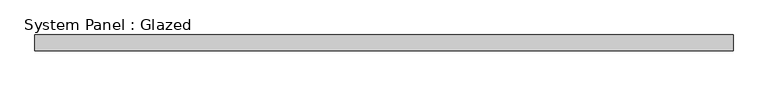
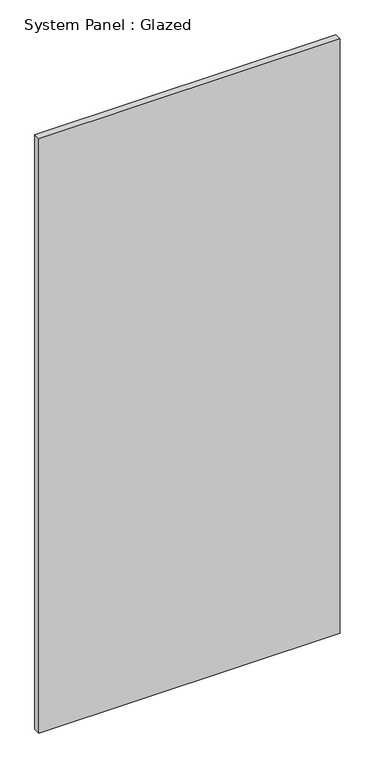
"""IFC4 building model written with IfcOpenShell, lengths in millimetres: plate geometry, System Panel : Glazed."""

from ifc_helpers import new_model, si_unit, origin, origin_with_axes, place, context, project, spatial, polyline, outline, extrude, source, transform, mapped, element, save


def system_panel_glazed_2148303e(model_context):
    return source(origin(), model_context, "Body", "SweptSolid", [
        extrude(outline(polyline([(561.975, 19.05), (-561.975, 19.05), (-561.975, 44.45), (561.975, 44.45), (561.975, 19.05)])), origin_with_axes(), (0.0, 0.0, 1.0), 2343.15),
    ])


if __name__ == "__main__":
    model = new_model("IFC4")
    model_context = context("Model", 3, world=origin())
    ifc_project = project(units=[si_unit("LENGTHUNIT", "METRE", prefix="MILLI")], contexts=[model_context])
    site = spatial("IfcSite", under=ifc_project)
    building = spatial("IfcBuilding", under=site)
    placement = place(None, origin())
    system_panel_glazed_shape = system_panel_glazed_2148303e(model_context)
    element("IfcPlate", 1, ObjectType="System Panel : Glazed", at=placement, inside=building, context=model_context, shape_type="MappedRepresentation", body=[
        mapped(system_panel_glazed_shape, transform((0.0, 0.0, 0.0), x_axis=(1.0, 0.0, 0.0), y_axis=(0.0, 1.0, 0.0), z_axis=(0.0, 0.0, 1.0))),
    ])
    save(model, "model.ifc")

# Revit data of these elements
# Type "System Panel : Glazed"
#   Construction Type Id = "GSP4R"
#   Analytic Construction = "1/8 in Pilkington single glazing"
#   Visual Light Transmittance = 0.9
#   Solar Heat Gain Coefficient = 0.86
#   Heat Transfer Coefficient (U) = 1.18115 BTU/(h·ft²·°F)
# Element 1 (IfcPlate, "System Panel : Glazed")
#   Materials on its faces: "Glass"
# Materials
#   "Glass": class "Glass", colour RGB 0 128 192, transparency 0.75, Description = "Soda Lime Glass", Cost = 0
